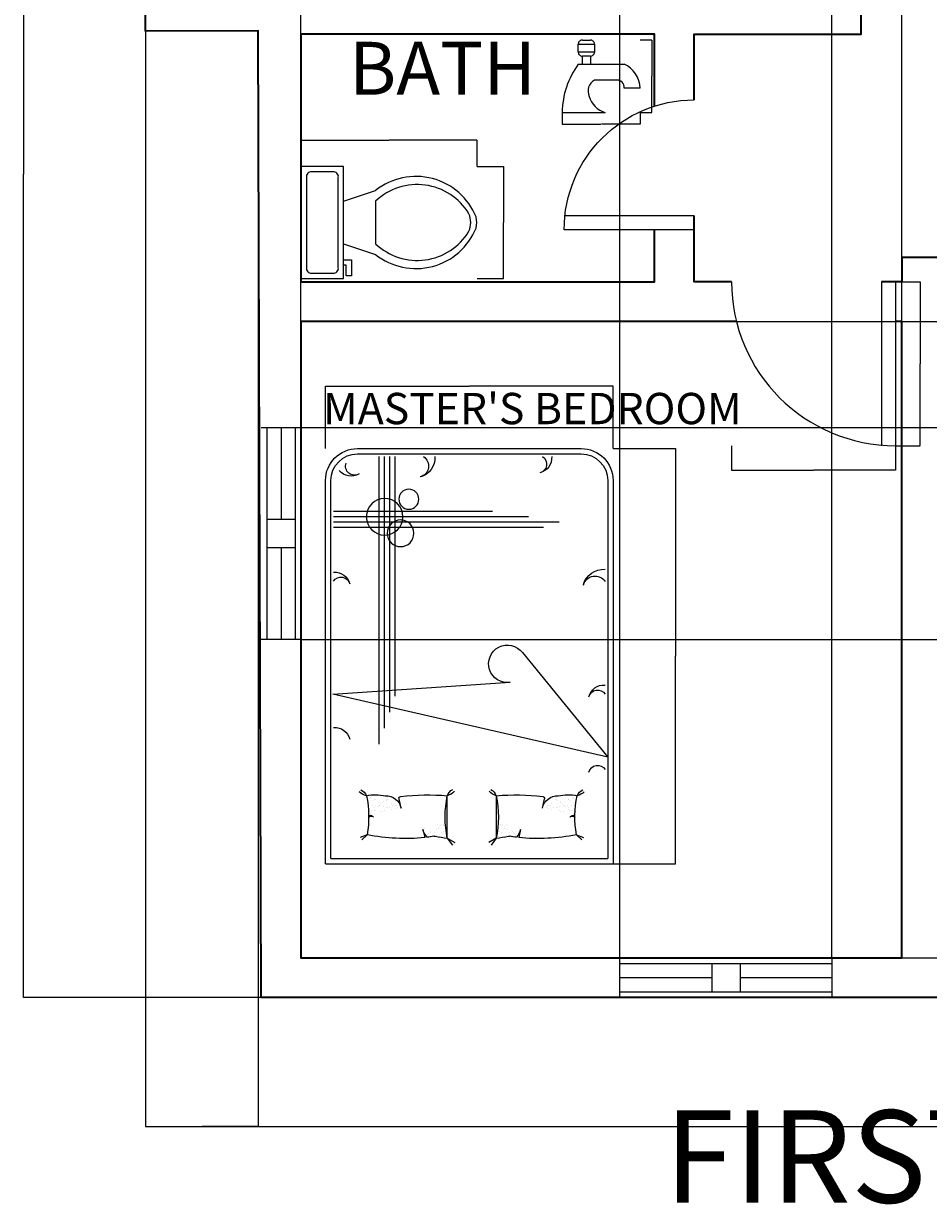
# Model space of a CAD drawing. Units: millimetres. Extents: x 19292 to 100733, y 12374 to 26974.
# Tile 19 of 24: x 42699 to 47819, y 12374 to 19054. Entities that reach past the tile are written whole.
import ezdxf

# ---------------------------------------------------------------- set-up
doc = ezdxf.new("R2010")
doc.units = ezdxf.units.MM
for name, color, linetype, lineweight in [('A-ANNO-DIMS', 2, 'Continuous', 18), ('A-ANNO-TEXT', 7, 'Continuous', 35), ('A-AREA-IDEN', 3, 'Continuous', 25), ('A-DOOR', 4, 'Continuous', 25), ('A-FLOR-FIXT', 9, 'Continuous', 18), ('A-FURN', 8, 'Continuous', 18), ('A-GLAZ', 3, 'Continuous', 25), ('A-WALL', 7, 'Continuous', 35)]:
    doc.layers.add(name, color=color, linetype=linetype, lineweight=lineweight)
doc.layers.add('FURNITURE', color=40, linetype='Continuous')
doc.layers.add('WINDOWS', color=50, linetype='Continuous')
doc.styles.get("Standard").update_dxf_attribs({"font": 'arial.ttf'})
doc.dimstyles.get("Standard").update_dxf_attribs({"dimtxt": 0.18, "dimasz": 0.18, "dimexe": 0.18, "dimexo": 0.0625, "dimgap": 0.09, "dimtad": 0, "dimtih": 1, "dimtoh": 1, "dimdec": 4, "dimzin": 0, "dimdsep": 46, "dimtxsty": 'Standard', "dimcen": 0.09, "dimadec": 0, "dimazin": 0, "dimtfac": 1, "dimtdec": 4, "dimtofl": 0, "dimtmove": 0, "dimatfit": 3, "dimfxl": 1, "dimtolj": 1, "dimtzin": 0, "dimarcsym": 0})

# ---------------------------------------------------------------- blocks, each defined once
blk = doc.blocks.new('DBED-4FT6')
at = {"layer": 'FURNITURE'}
for p, q in [((-27, 0), (-27, -72)), ((-27, 0), (26.99999999999997, 5.68e-14)), ((27, -72.00000000000023), (26.99999999999997, 5.68e-14)), ((-26, -1), (-26, -72)), ((-26, -1), (26.00000000000003, -0.9999999999997726)), ((26, -72.00000000000023), (26.00000000000003, -0.9999999999997726)), ((-4.134652103803261, -4.817063052123046), (-3.144796483066045, -3.500606371767958)), ((-4.134652103803261, -4.817063052122875), (-2.713769052616612, -3.999588591179417)), ((5.060678666421324, -4.817063052122875), (3.639795615234675, -3.999588591179417)), ((5.060678666421324, -4.817063052123046), (4.070823045684107, -3.500606371767958)), ((-19.18306202227052, -5.485972547936796), (-20.50060919072149, -4.967335516912726)), ((-19.18306202227052, -5.485972547936967), (-20.20772305100416, -4.498686779813965)), ((-8.713720467787255, -6.492365964457349), (-8.352181760678093, -4.952469549742318)), ((-8.40590424041818, -6.637378314066779), (-8.40590424041818, -6.637378314066779)), ((-8.239079784370745, -5.562538396824265), (-8.239079784370745, -5.562538396824265)), ((-7.82267294259384, -5.507717396091834), (-7.82267294259384, -5.507717396091834)), ((-7.611546033681406, -5.809807366600068), (-7.611546033681406, -5.809807366600068)), ((-7.515425131198753, -5.088011999378352), (-7.515425131198753, -5.088011999378352)), ((-7.374544898039516, -5.845988456355428), (-7.374544898039516, -5.845988456355428)), ((-7.367969663836447, -5.22313004090148), (-7.367969663836447, -5.22313004090148)), ((-7.274189455356292, -6.024727209938816), (-7.274189455356292, -6.024727209938816)), ((-6.736049374527851, -5.364660689418656), (-6.736049374527851, -5.364660689418656)), ((-6.571710140081449, -5.952767465126385), (-6.571710140081449, -5.952767465126385)), ((-6.245189668756381, -6.559531928114552), (-6.245189668756381, -6.559531928114552)), ((-6.085661545466621, -5.279035507322305), (-6.085661545466621, -5.279035507322305)), ((-5.875720334132552, -6.590524621115605), (-5.875720334132552, -6.590524621115605)), ((-5.669254703689716, -5.224214506589873), (-5.669254703689716, -5.224214506589873)), ((-5.280472006961815, -5.819278030439932), (-5.280472006961815, -5.819278030439932)), ((-5.120232544280042, -5.805280123770785), (-5.120232544280042, -5.805280123770785)), ((-4.782875965954929, -6.020199967109533), (-4.782875965954929, -6.020199967109533)), ((-4.582631135623728, -5.081157799916695), (-4.582631135623728, -5.081157799916695)), ((-4.249112664583094, -5.02788817272858), (-4.249112664583094, -5.02788817272858)), ((5.175139227201157, -5.027888172729319), (5.175139227201157, -5.027888172729319)), ((5.50865769824179, -5.081157799916638), (5.50865769824179, -5.081157799916638)), ((5.708902528572991, -6.020199967109817), (5.708902528572991, -6.020199967109817)), ((6.046259106898105, -5.805280123771126), (6.046259106898105, -5.805280123771126)), ((6.206498569579878, -5.819278030440671), (6.206498569579878, -5.819278030440671)), ((6.595281266307779, -5.224214506589817), (6.595281266307779, -5.224214506589817)), ((6.801746896750614, -6.590524621115321), (6.801746896750614, -6.590524621115321)), ((7.011688108084683, -5.279035507322305), (7.011688108084683, -5.279035507322305)), ((7.171216231373705, -6.559531928115234), (7.171216231373705, -6.559531928115234)), ((7.497736702698773, -5.952767465126157), (7.497736702698773, -5.952767465126157)), ((7.662075937145914, -5.364660689418599), (7.662075937145914, -5.364660689418599)), ((8.200216017975094, -6.024727209939328), (8.200216017975094, -6.024727209939328)), ((8.293996226453771, -5.223130040901196), (8.293996226453771, -5.223130040901196)), ((8.30057146065684, -5.84598845635628), (8.30057146065684, -5.84598845635628)), ((8.441451693816077, -5.088011999378068), (8.441451693816077, -5.088011999378068)), ((8.537572596300208, -5.80980736660058), (8.537572596300208, -5.80980736660058)), ((8.748699505211903, -5.507717396091777), (8.748699505211903, -5.507717396091777)), ((9.165106346988807, -5.562538396824265), (9.165106346988807, -5.562538396824265)), ((9.639747030405317, -6.492365964457349), (9.278208323295416, -4.952469549742318)), ((9.331930803035561, -6.637378314067632), (9.331930803035561, -6.637378314067632)), ((20.10908858488784, -5.485972547936967), (21.13374961362223, -4.498686779813965)), ((20.10908858488858, -5.485972547936796), (21.42663575333882, -4.967335516912726)), ((-5.998452499838663, -7.338874652100457), (-5.998452499838663, -7.338874652100457)), ((-5.728264866770928, -6.725642662638733), (-5.728264866770928, -6.725642662638733)), ((-5.688613537228434, -7.034850473630854), (-5.688613537228434, -7.034850473630854)), ((-5.348064670777432, -7.253249470004163), (-5.348064670777432, -7.253249470004163)), ((-5.230077320474265, -7.360737045650239), (-5.230077320474265, -7.360737045650239)), ((-4.93200534301593, -7.455280086863638), (-4.93200534301593, -7.455280086863638)), ((-4.931657828999789, -7.198428469271675), (-4.931657828999789, -7.198428469271675)), ((5.857684391617851, -7.198428469271505), (5.857684391617851, -7.198428469271505)), ((5.85803190563331, -7.455280086863353), (5.85803190563331, -7.455280086863353)), ((6.156103883091589, -7.360737045650921), (6.156103883091589, -7.360737045650921)), ((6.274091233394756, -7.253249470003993), (6.274091233394756, -7.253249470003993)), ((6.614640099846496, -7.034850473631365), (6.614640099846496, -7.034850473631365)), ((6.654291429388308, -6.725642662638449), (6.654291429388308, -6.725642662638449)), ((6.924479062455986, -7.338874652100287), (6.924479062455986, -7.338874652100287)), ((-18.77590810264172, -9.83900715250769), (-18.77590810264172, -9.83900715250769)), ((-18.7469186025819, -9.831933062623136), (-18.7469186025819, -9.831933062623136)), ((-18.59621655837128, -9.4634697248635), (-18.59621655837128, -9.4634697248635)), ((-18.43855152431661, -10.05392699584638), (-18.43855152431661, -10.05392699584638)), ((-18.181365058572, -11.01410595179413), (-18.181365058572, -11.01410595179413)), ((-17.90022675242233, -10.10122688085266), (-17.90022675242233, -10.10122688085266)), ((-17.75277128506002, -10.23634492237579), (-17.75277128506002, -10.23634492237579)), ((-17.73180625429978, -10.63313818015905), (-17.73180625429978, -10.63313818015905)), ((-17.53097722951077, -10.92848076969778), (-17.53097722951077, -10.92848076969778)), ((-17.11457038773386, -10.87365976896535), (-17.11457038773386, -10.87365976896535)), ((-16.95651176130502, -10.9659823466007), (-16.95651176130502, -10.9659823466007)), ((-16.85297560618875, -11.06405025953836), (-16.85297560618875, -11.06405025953836)), ((-16.70044691192106, -9.841748322447756), (-16.70044691192106, -9.841748322447756)), ((-16.2845946132411, -9.834479909678294), (-16.2845946132411, -9.834479909678294)), ((-16.02794681966861, -10.73060306229217), (-16.02794681966861, -10.73060306229217)), ((-15.94723803491598, -10.04939975301698), (-15.94723803491598, -10.04939975301698)), ((-15.57109168263798, -10.55529179420631), (-15.57109168263798, -10.55529179420631)), ((-15.37755899060738, -10.64497788019582), (-15.37755899060738, -10.64497788019582)), ((-14.96115214883048, -10.59015687946339), (-14.96115214883048, -10.59015687946339)), ((-14.55161047764721, -10.26384189465318), (-14.55161047764721, -10.26384189465318)), ((-14.36166211678738, -11.05952301670902), (-14.36166211678738, -11.05952301670902)), ((-13.87452858076449, -10.44710017279021), (-13.87452858076449, -10.44710017279021)), ((-13.85562067169906, -10.9015990506424), (-13.85562067169906, -10.9015990506424)), ((-13.70816520433675, -11.03671709216553), (-13.70816520433675, -11.03671709216553)), ((-13.52461999197714, -10.56510705403116), (-13.52461999197714, -10.56510705403116)), ((-12.80860301424707, -10.50441610444505), (-13.20654336081225, -12.19935747834682)), ((13.73462957686513, -10.50441610444505), (14.13256992343031, -12.19935747834682)), ((14.45064655459447, -10.56510705403201), (14.45064655459447, -10.56510705403201)), ((14.63419176695407, -11.03671709216536), (14.63419176695407, -11.03671709216536)), ((14.78164723431638, -10.90159905064223), (14.78164723431638, -10.90159905064223)), ((14.80055514338181, -10.44710017278998), (14.80055514338181, -10.44710017278998)), ((15.28768867940545, -11.05952301670942), (15.28768867940545, -11.05952301670942)), ((15.47763704026454, -10.26384189465307), (15.47763704026454, -10.26384189465307)), ((15.8871787114478, -10.59015687946316), (15.8871787114478, -10.59015687946316)), ((16.30358555322471, -10.64497788019565), (16.30358555322471, -10.64497788019565)), ((16.49711824525531, -10.55529179420722), (16.49711824525531, -10.55529179420722)), ((16.87326459753331, -10.04939975301738), (16.87326459753331, -10.04939975301738)), ((16.95397338228594, -10.73060306229195), (16.95397338228594, -10.73060306229195)), ((17.21062117585842, -9.834479909678635), (17.21062117585842, -9.834479909678635)), ((17.62647347453912, -9.841748322448382), (17.62647347453912, -9.841748322448382)), ((17.77900216880681, -11.06405025953882), (17.77900216880681, -11.06405025953882)), ((17.8825383239224, -10.96598234660052), (17.8825383239224, -10.96598234660052)), ((18.04059695035192, -10.87365976896512), (18.04059695035192, -10.87365976896512)), ((18.45700379212883, -10.92848076969761), (18.45700379212883, -10.92848076969761)), ((18.65783281691711, -10.63313818015967), (18.65783281691711, -10.63313818015967)), ((18.6787978476774, -10.23634492237556), (18.6787978476774, -10.23634492237556)), ((18.82625331503971, -10.10122688085243), (18.82625331503971, -10.10122688085243)), ((19.10739162119006, -11.01410595179391), (19.10739162119006, -11.01410595179391)), ((19.36457808693467, -10.05392699584672), (19.36457808693467, -10.05392699584672)), ((19.5222431209886, -9.463469724863273), (19.5222431209886, -9.463469724863273)), ((19.67294516519922, -9.831933062623932), (19.67294516519922, -9.831933062623932)), ((19.70193466525978, -9.839007152508032), (19.70193466525978, -9.839007152508032)), ((-18.69652391609435, -11.37339207783361), (-18.69652391609435, -11.37339207783361)), ((-18.66542323901467, -12.3058799545372), (-18.66542323901467, -12.3058799545372)), ((-18.6461292296068, -12.91485109304403), (-18.6461292296068, -12.91485109304403)), ((-18.51796777165236, -12.44099799606033), (-18.51796777165236, -12.44099799606033)), ((-18.12980541361923, -11.84228893838752), (-18.12980541361923, -11.84228893838752)), ((-17.79244883529407, -12.05720878172627), (-17.79244883529407, -12.05720878172627)), ((-17.68141156781223, -12.17459719536947), (-17.68141156781223, -12.17459719536947)), ((-17.44376818388207, -12.98831991447582), (-17.44376818388207, -12.98831991447582)), ((-16.79338035482089, -12.90269473237953), (-16.79338035482089, -12.90269473237953)), ((-16.65005222543351, -11.38320733765818), (-16.65005222543351, -11.38320733765818)), ((-16.59965753894596, -12.92466635286894), (-16.59965753894596, -12.92466635286894)), ((-16.37697351304393, -12.84787373164704), (-16.37697351304393, -12.84787373164704)), ((-16.26052195535686, -11.60373950258992), (-16.26052195535686, -11.60373950258992)), ((-16.11306648799456, -11.73885754411304), (-16.11306648799456, -11.73885754411304)), ((-15.63849192421787, -11.83776169555784), (-15.63849192421787, -11.83776169555784)), ((-15.52069699614969, -12.09675080941707), (-15.52069699614969, -12.09675080941707)), ((-15.31680696423956, -12.46849496833795), (-15.31680696423956, -12.46849496833795)), ((-15.3011353458927, -12.05268153889659), (-15.3011353458927, -12.05268153889659)), ((-15.29034994497795, -12.70481702497386), (-15.29034994497795, -12.70481702497386)), ((-14.55597933435581, -11.35649691174245), (-14.55597933435581, -11.35649691174245)), ((15.48200589697319, -11.35649691174331), (15.48200589697319, -11.35649691174331)), ((16.21637650759675, -12.70481702497392), (16.21637650759675, -12.70481702497392)), ((16.22716190851076, -12.05268153889693), (16.22716190851076, -12.05268153889693)), ((16.24283352685688, -12.46849496833772), (16.24283352685688, -12.46849496833772)), ((16.44672355876702, -12.09675080941792), (16.44672355876702, -12.09675080941792)), ((16.56451848683594, -11.83776169555824), (16.56451848683594, -11.83776169555824)), ((17.03909305061188, -11.73885754411276), (17.03909305061188, -11.73885754411276)), ((17.18654851797419, -11.60373950258963), (17.18654851797419, -11.60373950258963)), ((17.303000075662, -12.8478737316471), (17.303000075662, -12.8478737316471)), ((17.52568410156328, -12.92466635286979), (17.52568410156328, -12.92466635286979)), ((17.57607878805157, -11.38320733765908), (17.57607878805157, -11.38320733765908)), ((17.71940691743896, -12.90269473237953), (17.71940691743896, -12.90269473237953)), ((18.36979474650013, -12.98831991447588), (18.36979474650013, -12.98831991447588)), ((18.60743813042956, -12.17459719537038), (18.60743813042956, -12.17459719537038)), ((18.71847539791213, -12.05720878172661), (18.71847539791213, -12.05720878172661)), ((19.0558319762373, -11.84228893838792), (19.0558319762373, -11.84228893838792)), ((19.44399433426969, -12.4409979960601), (19.44399433426969, -12.4409979960601)), ((19.57215579222412, -12.91485109304494), (19.57215579222412, -12.91485109304494)), ((19.59144980163199, -12.30587995453698), (19.59144980163199, -12.30587995453698)), ((19.62255047871167, -11.37339207783429), (19.62255047871167, -11.37339207783429)), ((25.99999999999997, -20.04251490499428), (-25.62857142857144, -31.89664668985566)), ((9.968437092424097, -39.68281460107684), (25.99999999999997, -20.04251490499428)), ((-16.98298633143713, -76.49999999999977), (-16.98298633143804, -22.5)), ((-15.98298633143713, -76.49999999999977), (-15.98298633143804, -25.49999999999978)), ((-14.98298633143713, -76.49999999999977), (-14.98298633143804, -28.5)), ((-25.62857142857075, -31.89664668985566), (7.69367787486118, -34.10856123257989)), ((-13.98298633143713, -76.49999999999977), (-13.98298633143804, -31.5)), ((13.92237160184822, -63.18866900046464), (-25.5, -63.18866900046464)), ((16.878192650664, -64.18866900046464), (-25.5, -64.18866900046464)), ((11.10090459947105, -65.18866900046442), (-25.5, -65.18866900046464)), ((4.383130216417612, -66.18866900046442), (-25.5, -66.18866900046464)), ((-21, -77), (21, -77.0000000000002)), ((-21, -78), (21, -78.0000000000002))]:
    blk.add_line(p, q, dxfattribs=at)
for centre, radius in [((-12.91182106300494, -62.08454274520204), 2.504372971601696), ((-15.90739414396376, -65.18866900046464), 3.437232026160017), ((-11.36543750832788, -68.48173730478015), 1.878279728701272)]:
    blk.add_circle(centre, radius, dxfattribs=at)
for centre, radius, start, end in [((-39.10651142374138, -8.817063052122649), 20.20000000000147, 348.6069698988843, 9.491743103753544), ((-11.96490980142209, -41.81687628144138), 37.041008187906, 84.4028612645958, 101.2370836512883), ((-4.825879607851106, -7.608979000930446), 4.045013130436864, 139.9097590679286, 163.9755921234989), ((-11.52336853637479, -33.34663058587759), 28.57069839034993, 80.1409392097565, 82.7553866503384), ((-6.494365647111578, -4.409680956092984), 0.8, 260.1409392097565, 276.031827105606), ((-67.64177770808838, 360.6114736163754), 370.9058781068297, 279.5022474872839, 279.8588573948661), ((15.66534789619453, -8.817063052122135), 20.19999999999818, 168.5788137250011, 191.4211862750058), ((15.66534789619817, -8.817063052122649), 20.20000000000147, 168.5788137249941, 191.4211862750058), ((42751.26187429979, -8.817063056011648), 42755.39671351448, 179.9946396680611, 180.0053603319291), ((-14.73932133358011, -8.817063052122649), 20.20000000000147, 348.5788137249941, 11.42118627500586), ((-42750.33584773717, -8.817063056011648), 42755.39671351448, 359.9946396680676, 0.0053603319421324), ((-14.73932133357721, -8.817063052122135), 20.19999999999818, 348.5788137249941, 11.42118627499883), ((68.56780427070572, 360.6114736163754), 370.9058781068297, 260.141142605134, 260.4977525127162), ((7.420392209728902, -4.409680956092984), 0.8, 263.968172894394, 279.8590607902435), ((12.44939509899285, -33.34663058587759), 28.57069839034993, 97.2446133496616, 99.8590607902435), ((5.751906170469169, -7.608979000930446), 4.045013130436864, 16.0244078765011, 40.09024093207139), ((12.89093636403942, -41.81687628144138), 37.041008187906, 78.76291634871168, 95.59713873540417), ((40.03253798635941, -8.817063052122649), 20.20000000000147, 170.5082568962464, 191.3930301011157), ((-18.63439747950781, -8.362835026573748), 0.7823789253415179, 249.4968528373028, 325.7977956221763), ((-18.4002510232591, -8.445355047199143), 0.5460297530620258, 201.8040695959829, 319.1334346759098), ((19.32627758587716, -8.445355047199143), 0.5460297530620258, 220.8665653240902, 338.1959304040171), ((19.56042404212513, -8.362835026573748), 0.7823789253415179, 214.2022043778237, 290.5031471626973), ((-15.61384730787557, -9.916934814375791), 2.86610010521538, 266.7825255240543, 348.1719149754145), ((16.53987387049363, -9.916934814375791), 2.86610010521538, 191.8280850245854, 273.2174744759457), ((-18.77582684722529, -15.36188282958866), 2.608691937302173, 101.6935339662269, 136.5635486949323), ((-21.64959486574241, -11.66451602127745), 2.608691937302173, 299.1485263283325, 334.0185410570184), ((-17.59820796861624, -5.617120538590143), 7.389908305163763, 256.6498532633935, 284.285581023734), ((-12.81713200699761, -12.29078393797522), 0.4, 166.787330358343, 262.8769841008062), ((-7.849044883706142, 31.23309670203668), 44.20648468370187, 263.4825574665681, 274.8198866450032), ((-1.728460786103994, -11.80933443470422), 2.608691937302173, 202.7242534275457, 237.5942681562781), ((-4.807664589399962, -15.33744552666542), 2.608691937302173, 40.17924578964186, 75.04926051838007), ((5.733691152018025, -15.33744552666542), 2.608691937302173, 104.9507394816199, 139.8207542103581), ((2.654487348722057, -11.80933443470422), 2.608691937302173, 302.4057318437219, 337.2757465724543), ((8.775071446323466, 31.23309670203668), 44.20648468370187, 265.1801133549968, 276.5174425334318), ((13.74315856961567, -12.29078393797522), 0.4, 277.1230158991938, 13.21266964165692), ((18.52423453123356, -5.617120538590143), 7.389908305163763, 255.7144189762659, 283.3501467366066), ((19.70185340984335, -15.36188282958866), 2.608691937302173, 43.43645130506771, 78.3064660337731), ((22.57562142836048, -11.66451602127745), 2.608691937302173, 205.9814589429815, 240.8514736716675), ((24.08149477166717, -16.81385886181465), 1.693091563593251, 194.451540940981, 326.9105817271671), ((-25.2881588087821, -22.70588367900495), 2.933920970030247, 265.8594053605621, 345.9527428336846), ((24.08149477166717, -30.96393635208892), 1.693091563593251, 194.451540940981, 326.9105817271671), ((25.28815880878119, -30.6743386403075), 2.933920970030691, 194.0472571663257, 274.140594639438), ((7.144201548013711, -37.58406550475044), 3.518672218272346, 81.0159135592615, 323.3831798465962), ((-25.28815880878119, -51.86055593582091), 2.933920970030691, 265.8594053605621, 345.9527428336743), ((-24.08149477166717, -52.15015364760233), 1.693091563593251, 213.0894182728328, 345.548459059019), ((23.60865969555653, -51.81050935983859), 2.257455418124377, 194.451540940981, 326.9105817271699), ((25.21754507837523, -51.42437907746352), 3.911894626707589, 194.0472571663257, 274.140594639438), ((-21, -72), 6, 180, 270), ((-21, -72), 5, 180, 270), ((-22.19032021997464, -75.74024097389656), 2.933920970030691, 59.04725716631266, 140.6216534048161), ((-21.541856402534, -74.6822241448225), 1.69309156359317, 59.45154094095176, 200.6983000057678), ((-9.760470192471985, -74.7268684645835), 2.116364454491481, 303.0894182728446, 75.5484590590127), ((-10.12246733219854, -76.23519851097626), 3.667401212538364, 355.8594053605848, 75.95274283367745), ((21, -72.00000000000023), 5, 270, 0), ((21, -72.00000000000023), 6, 270, 0), ((12.54583364175596, -76.28815880878142), 2.933920970030691, 355.8594053605848, 75.95274283367745), ((12.83543135353738, -75.081494771667), 1.693091563593251, 303.0894182728446, 75.5484590590127)]:
    blk.add_arc(centre, radius, start, end, dxfattribs=at)
blk = doc.blocks.new('TAP-SIDELEV')
for p, q in [((0.9999853785046433, 4.25000541523623), (1.999985378504643, 4.25000541523623)), ((1.999985378504643, 3.75000541523623), (0.9999853785046433, 3.75000541523623)), ((0.9999853785046433, 3.00000541523623), (3.840125540729427, 3.00000541523623)), ((1.249985378504643, 3.00000541523623), (1.249985378504643, 3.50000541523623)), ((1.749985378504643, 3.50000541523623), (1.749985378504643, 3.00000541523623)), ((3.527288395467852, 2.00000541523623), (1.999985378504643, 2.00000541523623)), ((4.840309954143972, 1.50000541523623), (3.840309954143972, 1.50000541523623)), ((-1.46214953567e-05, 5.415236231e-06), (0.2499853785046433, 5.415236231e-06)), ((0.2499853785046433, 5.415236231e-06), (2.675565113506539, 5.415236231e-06))]:
    blk.add_line(p, q)
for points in [[(1.249985378504643, 4.50000541523623), (1.749985378504643, 4.50000541523623)], [(0.9999853785046433, 3.75000541523623), (0.9999853785046433, 4.25000541523623)], [(1.999985378504643, 4.25000541523623), (1.999985378504643, 3.75000541523623)], [(1.749985378504643, 3.50000541523623), (1.249985378504643, 3.50000541523623)]]:
    blk.add_lwpolyline(points)
for centre, radius, start, end in [((1.242385378504675, 4.257505415236281), 0.2425917, 88.22243000000017, 181.7776), ((1.757485378504636, 4.257505415236281), 0.2425917, 358.2224, 91.77756999999983), ((1.242385378504675, 3.742405415236319), 0.2425917, 178.2223999999999, 271.7775999999998), ((1.757485378504636, 3.742405415236319), 0.2425917, 268.2224000000001, 1.777565000000075), ((5.084285378504628, -0.0280945847637639), 5.084362999999999, 143.4467, 179.6834000000001), ((3.172409954143997, 1.471305415236273), 1.668163, 0.9827694999999721, 66.40494208784), ((2.37686141733268, 1.325114461238403), 0.7729898760208992, 119.180086595352, 204.871573560288), ((3.433909954144009, 1.593605415236268), 0.4169898, 347.0191999999999, 102.9807999999998), ((3.050564044119678, 1.37500541523623), 1.425219, 195.2551000000002, 254.7449000000001)]:
    blk.add_arc(centre, radius, start, end)
blk = doc.blocks.new('WC01')
at = {"layer": 'FURNITURE'}
for p, q in [((10.5, 0), (-10.5, 0)), ((-10.5, 0), (-10.5, -8)), ((10.5, -8), (10.5, 0)), ((-9.5, -2), (-9.5, -6)), ((8.5, -1), (-8.5, -1)), ((9.5, -6), (9.5, -2)), ((-10.5, -8), (10.5, -8)), ((-10, -9.5), (-10, -8.5)), ((-10, -8.5), (-8, -8.5)), ((-8.5, -7), (8.5, -7)), ((-8, -8.5), (-8, -8)), ((-7, -8), (-7, -9.5)), ((-4, -8), (-6, -14)), ((4, -8), (6, -14)), ((-7, -9.5), (-10, -9.5)), ((4, -14), (-4, -14))]:
    blk.add_line(p, q, dxfattribs=at)
for centre, radius, start, end in [((-8.625, -1.875), 0.8838834999999999, 81.86989999999966, 188.1301000000003), ((8.625, -1.875), 0.8838834999999999, 351.8698999999996, 98.13010000000035), ((-8.625, -6.125), 0.8838834999999999, 171.8698980000006, 278.1301000000004), ((8.625, -6.125), 0.8838834999999999, 261.8698999999996, 8.13010000000033), ((3.519562435188959, -21.58049502388982), 12.16902005083646, 141.4691096810951, 247.9714346835572), ((4.199957580658804, -21.81740929088454), 11.3291791325804, 136.3677254423712, 238.9468239374052), ((-3.519499936778316, -21.58047137067521), 12.16903423757823, 292.0284332733146, 38.5307063680049), ((-4.199890672038463, -21.81738596564128), 11.32918622148567, 301.0530065773862, 43.6320921669473), ((2.09660981625e-05, -27.87646475467881), 4, 245.7318247449368, 294.2681740488958), ((2.09415214272e-05, -28.99996806116076), 4, 254.8605283244431, 285.1394707718437)]:
    blk.add_arc(centre, radius, start, end, dxfattribs=at)
blk = doc.blocks.new('WW')
at = {"layer": 'WINDOWS'}
for p, q in [((-5183.867826392408, -4940.876860268414), (-3983.867826392409, -4940.876860268414)), ((-4663.867826392415, -4940.876860268414), (-4663.867826392408, -5100.876860268415)), ((-4503.867826392416, -4940.876860268414), (-4503.867826392408, -5100.876860268415)), ((-4503.867826392416, -4940.876860268414), (-4503.867826392408, -5100.876860268415)), ((-5183.867826392408, -5020.876860268414), (-4663.867826392408, -5020.876860268415)), ((-4503.867826392416, -5020.876860268414), (-3983.867826392409, -5020.876860268414)), ((-5183.867826392408, -5100.876860268414), (-3983.867826392409, -5100.876860268414))]:
    blk.add_line(p, q, dxfattribs=at)
for points in [[(-5183.867826392408, -5133.376860268413), (-5183.867826392408, -4908.376860268414)], [(-3983.867826392409, -4908.376860268414), (-3983.867826392409, -5133.376860268413)]]:
    blk.add_lwpolyline(points, dxfattribs=at)
blk = doc.blocks.new('DOOR-750')
for p, q in [((655.272448405085, -6.32018709439e-05), (655.272448405085, 735.2719952907646)), ((735.272448405085, -6.32018709439e-05), (735.272448405085, 735.2719952907646)), ((735.272448405085, -6.32018709439e-05), (655.272448405085, -6.32018709439e-05)), ((735.272448405085, -6.32018709439e-05), (655.272448405085, -6.32018709439e-05))]:
    blk.add_line(p, q)
blk.add_arc((735.272448405085, -6.32018709439e-05), 735.2720584926371, 90, 180)
blk = doc.blocks.new('DOOR-SWING-900')
blk.add_line((927.6985029579554, 927.698603252542), (927.6985029579554, -0.0001625114309718))
blk.add_arc((927.6985029579554, 927.698603252542), 927.6987657639734, 180, 270)
blk = doc.blocks.new('*D24')
at = {"layer": 'A-ANNO-DIMS', "color": 0, "lineweight": -2, "transparency": 16777216}
for p, q in [((46034.63806935272, 16650.17552620515), (46387.30813187039, 16650.17552620515)), ((46387.12813187039, 16649.99552620515), (46387.1281318704, 15475.1835101731)), ((46387.1281318704, 14300.00510942071), (46387.1281318704, 15474.81712545277)), ((46034.63806935272, 14299.82510942071), (46387.3081318704, 14299.82510942071))]:
    blk.add_line(p, q, dxfattribs=at)
at = {"layer": 'A-ANNO-DIMS', "color": 0, "transparency": 16777216}
for points in [[(46387.09813187039, 16649.99552620515), (46387.15813187038, 16649.99552620515), (46387.12813187039, 16650.17552620515)], [(46387.09813187039, 14300.00510942071), (46387.15813187039, 14300.00510942071), (46387.1281318704, 14299.82510942071)]]:
    blk.add_solid(points, dxfattribs=at)
at = {"layer": 'Defpoints', "color": 0, "transparency": 16777216}
for p in [(46034.57556935271, 16650.17552620515), (46034.57556935271, 14299.82510942071), (46387.1281318704, 14299.82510942071)]:
    blk.add_point(p, dxfattribs=at)
at = {"layer": 'A-ANNO-DIMS', "color": 0, "transparency": 16777216, "insert": (46387.12813187039, 15475.00031781291), "char_height": 0.18, "attachment_point": 5}
blk.add_mtext('\\A1;DOUBLE BED 2350 TYP.', dxfattribs=at)
blk = doc.blocks.new('*D25')
at = {"layer": 'A-ANNO-DIMS', "color": 0, "lineweight": -2, "transparency": 16777216}
for p, q in [((44407.40989619425, 16650.23802620514), (44407.40989619425, 17002.90808872281)), ((44407.58989619425, 17002.72808872281), (45220.3332648335, 17002.72808872281)), ((46034.3955693527, 17002.72808872281), (45221.65220071345, 17002.72808872281)), ((46034.5755693527, 16650.23802620514), (46034.5755693527, 17002.90808872281))]:
    blk.add_line(p, q, dxfattribs=at)
at = {"layer": 'A-ANNO-DIMS', "color": 0, "transparency": 16777216}
for points in [[(44407.58989619425, 17002.75808872281), (44407.58989619425, 17002.69808872281), (44407.40989619425, 17002.72808872281)], [(46034.3955693527, 17002.75808872281), (46034.3955693527, 17002.69808872281), (46034.5755693527, 17002.72808872281)]]:
    blk.add_solid(points, dxfattribs=at)
at = {"layer": 'Defpoints', "color": 0, "transparency": 16777216}
for p in [(46034.5755693527, 17002.72808872281), (44407.40989619425, 16650.17552620514), (46034.5755693527, 16650.17552620514)]:
    blk.add_point(p, dxfattribs=at)
at = {"layer": 'A-ANNO-DIMS', "color": 0, "transparency": 16777216, "insert": (45220.99273277348, 17002.72808872281), "char_height": 0.18, "attachment_point": 5}
blk.add_mtext('\\A1;1627 TYP.', dxfattribs=at)
blk = doc.blocks.new('*D28')
at = {"layer": 'A-ANNO-DIMS', "color": 0, "lineweight": -2, "transparency": 16777216}
for p, q in [((47632.94877694873, 17593.99260027244), (47772.22109181335, 17593.99260027244)), ((47772.04109181335, 17593.81260027244), (47772.04109181335, 17130.32634835907)), ((47772.04109181335, 16666.47383450846), (47772.04109181335, 17129.96008642183)), ((47632.94877694873, 16666.29383450846), (47772.22109181335, 16666.29383450846))]:
    blk.add_line(p, q, dxfattribs=at)
at = {"layer": 'A-ANNO-DIMS', "color": 0, "transparency": 16777216}
for points in [[(47772.01109181334, 17593.81260027244), (47772.07109181334, 17593.81260027244), (47772.04109181335, 17593.99260027244)], [(47772.01109181334, 16666.47383450846), (47772.07109181334, 16666.47383450846), (47772.04109181335, 16666.29383450846)]]:
    blk.add_solid(points, dxfattribs=at)
at = {"layer": 'Defpoints', "color": 0, "transparency": 16777216}
for p in [(47632.88627694873, 17593.99260027244), (47772.04109181335, 17593.99260027244), (47632.88627694873, 16666.29383450846)]:
    blk.add_point(p, dxfattribs=at)
at = {"layer": 'A-ANNO-DIMS', "color": 0, "transparency": 16777216, "insert": (47772.04109181335, 17130.14321739043), "char_height": 0.18, "attachment_point": 5}
blk.add_mtext('\\A1;DOOR 900 928 TYP.', dxfattribs=at)
blk = doc.blocks.new('*D29')
at = {"layer": 'A-ANNO-DIMS', "color": 0, "lineweight": -2, "transparency": 16777216}
for p, q in [((46705.18751118475, 16666.23133450846), (46705.18751118475, 16526.95901964386)), ((47632.88627694872, 16666.23133450846), (47632.88627694872, 16526.95901964386)), ((46705.36751118476, 16527.13901964386), (47168.43887905992, 16527.13901964386)), ((47632.70627694871, 16527.13901964386), (47169.63490907356, 16527.13901964386))]:
    blk.add_line(p, q, dxfattribs=at)
at = {"layer": 'A-ANNO-DIMS', "color": 0, "transparency": 16777216}
for points in [[(46705.36751118476, 16527.16901964386), (46705.36751118476, 16527.10901964386), (46705.18751118475, 16527.13901964386)], [(47632.70627694871, 16527.16901964386), (47632.70627694871, 16527.10901964386), (47632.88627694872, 16527.13901964386)]]:
    blk.add_solid(points, dxfattribs=at)
at = {"layer": 'Defpoints', "color": 0, "transparency": 16777216}
for p in [(46705.18751118475, 16666.29383450846), (47632.88627694872, 16666.29383450846), (47632.88627694872, 16527.13901964386)]:
    blk.add_point(p, dxfattribs=at)
at = {"layer": 'A-ANNO-DIMS', "color": 0, "transparency": 16777216, "insert": (47169.03689406674, 16527.13901964386), "char_height": 0.18, "attachment_point": 5}
blk.add_mtext('\\A1;928 TYP.', dxfattribs=at)
blk = doc.blocks.new('*D38')
at = {"layer": 'A-ANNO-DIMS', "color": 0, "lineweight": -2, "transparency": 16777216}
for p, q in [((44268.67420168258, 18245.59675392526), (44268.67420168258, 18395.08012642252)), ((44268.85420168257, 18394.90012642252), (44765.71434511363, 18394.90012642252)), ((45264.26668499762, 18394.90012642252), (44767.40654156657, 18394.90012642252)), ((45264.44668499763, 18245.59675392526), (45264.44668499763, 18395.08012642252))]:
    blk.add_line(p, q, dxfattribs=at)
at = {"layer": 'A-ANNO-DIMS', "color": 0, "transparency": 16777216}
for points in [[(44268.85420168257, 18394.93012642252), (44268.85420168257, 18394.87012642252), (44268.67420168258, 18394.90012642252)], [(45264.26668499762, 18394.93012642252), (45264.26668499762, 18394.87012642252), (45264.44668499763, 18394.90012642252)]]:
    blk.add_solid(points, dxfattribs=at)
at = {"layer": 'Defpoints', "color": 0, "transparency": 16777216}
for p in [(44268.67420168258, 18394.90012642252), (44268.67420168258, 18245.53425392526), (45264.44668499763, 18245.53425392526)]:
    blk.add_point(p, dxfattribs=at)
at = {"layer": 'A-ANNO-DIMS', "color": 0, "transparency": 16777216, "insert": (44766.5604433401, 18394.90012642252), "char_height": 0.18, "attachment_point": 5}
blk.add_mtext('\\A1;WC 996 TYP.', dxfattribs=at)
blk = doc.blocks.new('*D39')
at = {"layer": 'A-ANNO-DIMS', "color": 0, "lineweight": -2, "transparency": 16777216}
for p, q in [((45264.50918499764, 18245.53425392527), (45413.99255749491, 18245.53425392527)), ((45413.81255749492, 18245.35425392527), (45413.81255749492, 17929.32289311824)), ((45413.81255749492, 17612.92760325254), (45413.81255749492, 17928.95896405957)), ((45264.50918499764, 17612.74760325254), (45413.99255749491, 17612.74760325254))]:
    blk.add_line(p, q, dxfattribs=at)
at = {"layer": 'A-ANNO-DIMS', "color": 0, "transparency": 16777216}
for points in [[(45413.78255749491, 18245.35425392527), (45413.84255749491, 18245.35425392527), (45413.81255749492, 18245.53425392527)], [(45413.78255749491, 17612.92760325254), (45413.84255749491, 17612.92760325254), (45413.81255749492, 17612.74760325254)]]:
    blk.add_solid(points, dxfattribs=at)
at = {"layer": 'Defpoints', "color": 0, "transparency": 16777216}
for p in [(45264.44668499764, 18245.53425392527), (45413.81255749492, 18245.53425392527), (45264.44668499764, 17612.74760325254)]:
    blk.add_point(p, dxfattribs=at)
at = {"layer": 'A-ANNO-DIMS', "color": 0, "transparency": 16777216, "insert": (45413.81255749492, 17929.14092858889), "char_height": 0.18, "attachment_point": 5}
blk.add_mtext('\\A1;633 TYP.', dxfattribs=at)
blk = doc.blocks.new('*D40')
at = {"layer": 'A-ANNO-DIMS', "color": 0, "lineweight": -2, "transparency": 16777216}
for p, q in [((45746.8110979714, 18551.75783262261), (45746.8110979714, 18485.54556456821)), ((46187.44288500068, 18551.75783262261), (46187.44288500068, 18485.54556456821)), ((45746.9910979714, 18485.72556456821), (45965.70092736599, 18485.72556456821)), ((46187.26288500068, 18485.72556456821), (45968.5530556061, 18485.72556456821))]:
    blk.add_line(p, q, dxfattribs=at)
at = {"layer": 'A-ANNO-DIMS', "color": 0, "transparency": 16777216}
for points in [[(45746.9910979714, 18485.75556456821), (45746.9910979714, 18485.69556456822), (45746.8110979714, 18485.72556456821)], [(46187.26288500068, 18485.75556456821), (46187.26288500068, 18485.69556456822), (46187.44288500068, 18485.72556456821)]]:
    blk.add_solid(points, dxfattribs=at)
at = {"layer": 'Defpoints', "color": 0, "transparency": 16777216}
for p in [(45746.8110979714, 18551.82033262261), (46187.44288500068, 18551.82033262261), (46187.44288500068, 18485.72556456821)]:
    blk.add_point(p, dxfattribs=at)
at = {"layer": 'A-ANNO-DIMS', "color": 0, "transparency": 16777216, "insert": (45967.12699148604, 18485.72556456821), "char_height": 0.18, "attachment_point": 5}
blk.add_mtext('\\A1;WASH BASIN 441 TYP.', dxfattribs=at)
blk = doc.blocks.new('*D41')
at = {"layer": 'A-ANNO-DIMS', "color": 0, "lineweight": -2, "transparency": 16777216}
for p, q in [((46187.5053850007, 18961.65695604733), (46253.7176530551, 18961.65695604733)), ((46253.53765305511, 18961.47695604733), (46253.53765305511, 18756.92054747276)), ((46253.53765305511, 18552.00033262262), (46253.53765305511, 18756.55674119719)), ((46187.5053850007, 18551.82033262262), (46253.7176530551, 18551.82033262262))]:
    blk.add_line(p, q, dxfattribs=at)
at = {"layer": 'A-ANNO-DIMS', "color": 0, "transparency": 16777216}
for points in [[(46253.50765305511, 18961.47695604733), (46253.5676530551, 18961.47695604733), (46253.53765305511, 18961.65695604733)], [(46253.50765305511, 18552.00033262262), (46253.5676530551, 18552.00033262262), (46253.53765305511, 18551.82033262262)]]:
    blk.add_solid(points, dxfattribs=at)
at = {"layer": 'Defpoints', "color": 0, "transparency": 16777216}
for p in [(46187.4428850007, 18961.65695604733), (46253.53765305511, 18961.65695604733), (46187.4428850007, 18551.82033262262)]:
    blk.add_point(p, dxfattribs=at)
at = {"layer": 'A-ANNO-DIMS', "color": 0, "transparency": 16777216, "insert": (46253.53765305511, 18756.73864433496), "char_height": 0.18, "attachment_point": 5}
blk.add_mtext('\\A1;410 TYP.', dxfattribs=at)
blk = doc.blocks.new('*D100')
at = {"layer": 'A-ANNO-DIMS', "color": 0, "lineweight": -2, "transparency": 16777216}
for p, q in [((43388.92950300001, 22860.72493700001), (42698.81200300003, 22860.72493700001)), ((42698.99200300002, 22860.54493700001), (42698.99200300002, 18202.54073302934)), ((42698.99200300003, 13544.17260000001), (42698.99200300002, 18202.17680397067)), ((44043.61170200002, 13543.9926), (42698.81200300003, 13543.9926))]:
    blk.add_line(p, q, dxfattribs=at)
at = {"layer": 'A-ANNO-DIMS', "color": 0, "transparency": 16777216}
for points in [[(42698.96200300003, 22860.54493700001), (42699.02200300003, 22860.54493700001), (42698.99200300002, 22860.72493700001)], [(42698.96200300004, 13544.17260000001), (42699.02200300003, 13544.17260000001), (42698.99200300003, 13543.9926)]]:
    blk.add_solid(points, dxfattribs=at)
at = {"layer": 'Defpoints', "color": 0, "transparency": 16777216}
for p in [(43388.99200300001, 22860.72493700001), (42698.99200300003, 13543.9926), (44043.67420200001, 13543.9926)]:
    blk.add_point(p, dxfattribs=at)
at = {"layer": 'A-ANNO-DIMS', "color": 0, "transparency": 16777216, "insert": (42698.99200300002, 18202.35876849999), "char_height": 0.18, "attachment_point": 5}
blk.add_mtext('\\A1;9317', dxfattribs=at)
blk = doc.blocks.new('*D103')
at = {"layer": 'A-ANNO-DIMS', "color": 0, "lineweight": -2, "transparency": 16777216}
for p, q in [((44268.04262900001, 15568.9926), (57530.22278900005, 15568.99260000001)), ((57530.04278900005, 15568.81260000001), (57530.04278900005, 14669.1745031378)), ((57530.04278900005, 13769.17260000001), (57530.04278900005, 14668.81069686222)), ((44268.04262900001, 13768.9926), (57530.22278900005, 13768.99260000001))]:
    blk.add_line(p, q, dxfattribs=at)
at = {"layer": 'A-ANNO-DIMS', "color": 0, "transparency": 16777216}
for points in [[(57530.01278900006, 15568.81260000001), (57530.07278900005, 15568.81260000001), (57530.04278900005, 15568.99260000001)], [(57530.01278900006, 13769.17260000001), (57530.07278900005, 13769.17260000001), (57530.04278900005, 13768.99260000001)]]:
    blk.add_solid(points, dxfattribs=at)
at = {"layer": 'Defpoints', "color": 0, "transparency": 16777216}
for p in [(44267.98012900001, 15568.9926), (57530.04278900005, 15568.99260000001), (44267.98012900001, 13768.9926)]:
    blk.add_point(p, dxfattribs=at)
at = {"layer": 'A-ANNO-DIMS', "color": 0, "transparency": 16777216, "insert": (57530.04278900004, 14668.99259999999), "char_height": 0.18, "attachment_point": 5}
blk.add_mtext('\\A1;1800', dxfattribs=at)
blk = doc.blocks.new('*D104')
at = {"layer": 'A-ANNO-DIMS', "color": 0, "lineweight": -2, "transparency": 16777216}
for p, q in [((44268.04262900001, 17368.99260000001), (57530.22278900005, 17368.99260000001)), ((57530.04278900005, 17368.81260000001), (57530.04278900005, 17069.1745031378)), ((57530.04278900005, 16769.17260000001), (57530.04278900005, 17068.81069686222)), ((44268.04262900001, 16768.99260000001), (57530.22278900005, 16768.99260000001))]:
    blk.add_line(p, q, dxfattribs=at)
at = {"layer": 'A-ANNO-DIMS', "color": 0, "transparency": 16777216}
for points in [[(57530.01278900006, 17368.81260000001), (57530.07278900005, 17368.81260000001), (57530.04278900005, 17368.99260000001)], [(57530.01278900006, 16769.17260000001), (57530.07278900005, 16769.17260000001), (57530.04278900005, 16768.99260000001)]]:
    blk.add_solid(points, dxfattribs=at)
at = {"layer": 'Defpoints', "color": 0, "transparency": 16777216}
for p in [(44267.98012900001, 17368.99260000001), (57530.04278900005, 17368.99260000001), (44267.98012900001, 16768.99260000001)]:
    blk.add_point(p, dxfattribs=at)
at = {"layer": 'A-ANNO-DIMS', "color": 0, "transparency": 16777216, "insert": (57530.04278900005, 17068.99259999999), "char_height": 0.18, "attachment_point": 5}
blk.add_mtext('\\A1;600', dxfattribs=at)
blk = doc.blocks.new('*D112')
at = {"layer": 'A-ANNO-DIMS', "color": 0, "lineweight": -2, "transparency": 16777216}
for p, q in [((43388.992003, 22860.662437), (43388.992003, 12813.8126)), ((56840.04278899999, 15985.662601), (56840.04278899999, 12813.8126)), ((43389.172003, 12813.9926), (50114.11454470395, 12813.9926)), ((56839.86278899999, 12813.9926), (50114.92024729603, 12813.9926))]:
    blk.add_line(p, q, dxfattribs=at)
at = {"layer": 'A-ANNO-DIMS', "color": 0, "transparency": 16777216}
for points in [[(43389.172003, 12814.0226), (43389.172003, 12813.9626), (43388.992003, 12813.9926)], [(56839.86278899999, 12814.0226), (56839.86278899999, 12813.9626), (56840.04278899999, 12813.9926)]]:
    blk.add_solid(points, dxfattribs=at)
at = {"layer": 'Defpoints', "color": 0, "transparency": 16777216}
for p in [(43388.992003, 22860.724937), (56840.04278899999, 15985.725101), (56840.04278899999, 12813.9926)]:
    blk.add_point(p, dxfattribs=at)
at = {"layer": 'A-ANNO-DIMS', "color": 0, "transparency": 16777216, "insert": (50114.517396, 12813.9926), "char_height": 0.18, "attachment_point": 5}
blk.add_mtext('\\A1;13451', dxfattribs=at)
blk = doc.blocks.new('*D113')
at = {"layer": 'A-ANNO-DIMS', "color": 0, "lineweight": -2, "transparency": 16777216}
for p, q in [((43388.992003, 19010.662437), (43388.992003, 12813.8126)), ((44026.778429, 19012.632903), (44026.778429, 12813.8126)), ((43389.172003, 12813.9926), (43707.49083673669, 12813.9926)), ((44026.598429, 12813.9926), (43708.27959526329, 12813.9926))]:
    blk.add_line(p, q, dxfattribs=at)
at = {"layer": 'A-ANNO-DIMS', "color": 0, "transparency": 16777216}
for points in [[(43389.172003, 12814.0226), (43389.172003, 12813.9626), (43388.992003, 12813.9926)], [(44026.598429, 12814.0226), (44026.598429, 12813.9626), (44026.778429, 12813.9926)]]:
    blk.add_solid(points, dxfattribs=at)
at = {"layer": 'Defpoints', "color": 0, "transparency": 16777216}
for p in [(43388.992003, 19010.724937), (44026.778429, 19012.695403), (44026.778429, 12813.9926)]:
    blk.add_point(p, dxfattribs=at)
at = {"layer": 'A-ANNO-DIMS', "color": 0, "transparency": 16777216, "insert": (43707.88521599999, 12813.9926), "char_height": 0.18, "attachment_point": 5}
blk.add_mtext('\\A1;637.8', dxfattribs=at)
blk = doc.blocks.new('*D114')
at = {"layer": 'A-ANNO-DIMS', "color": 0, "lineweight": -2, "transparency": 16777216}
for p, q in [((44267.980129, 13769.0551), (44267.980129, 23550.904937)), ((44268.160129, 23550.724937), (45170.14306305662, 23550.724937)), ((46072.82794799999, 23550.724937), (45170.84501394339, 23550.724937)), ((46073.007948, 13769.0551), (46073.007948, 23550.904937))]:
    blk.add_line(p, q, dxfattribs=at)
at = {"layer": 'A-ANNO-DIMS', "color": 0, "transparency": 16777216}
for points in [[(44268.160129, 23550.754937), (44268.160129, 23550.694937), (44267.980129, 23550.724937)], [(46072.82794799999, 23550.754937), (46072.82794799999, 23550.694937), (46073.007948, 23550.724937)]]:
    blk.add_solid(points, dxfattribs=at)
at = {"layer": 'Defpoints', "color": 0, "transparency": 16777216}
for p in [(46073.007948, 23550.724937), (44267.980129, 13768.9926), (46073.007948, 13768.9926)]:
    blk.add_point(p, dxfattribs=at)
at = {"layer": 'A-ANNO-DIMS', "color": 0, "transparency": 16777216, "insert": (45170.4940385, 23550.724937), "char_height": 0.18, "attachment_point": 5}
blk.add_mtext('\\A1;1805', dxfattribs=at)
blk = doc.blocks.new('*D115')
at = {"layer": 'A-ANNO-DIMS', "color": 0, "lineweight": -2, "transparency": 16777216}
for p, q in [((47273.00794799999, 13769.0551), (47273.00794799999, 23550.904937)), ((47273.187948, 23550.724937), (47470.2045773813, 23550.724937)), ((47667.800129, 23550.724937), (47470.78349961869, 23550.724937)), ((47667.980129, 13769.0551), (47667.980129, 23550.904937))]:
    blk.add_line(p, q, dxfattribs=at)
at = {"layer": 'A-ANNO-DIMS', "color": 0, "transparency": 16777216}
for points in [[(47273.187948, 23550.754937), (47273.187948, 23550.694937), (47273.00794799999, 23550.724937)], [(47667.800129, 23550.754937), (47667.800129, 23550.694937), (47667.980129, 23550.724937)]]:
    blk.add_solid(points, dxfattribs=at)
at = {"layer": 'Defpoints', "color": 0, "transparency": 16777216}
for p in [(47667.980129, 23550.724937), (47273.00794799999, 13768.9926), (47667.980129, 13768.9926)]:
    blk.add_point(p, dxfattribs=at)
at = {"layer": 'A-ANNO-DIMS', "color": 0, "transparency": 16777216, "insert": (47470.4940385, 23550.724937), "char_height": 0.18, "attachment_point": 5}
blk.add_mtext('\\A1;395', dxfattribs=at)

msp = doc.modelspace()

# ---------------------------------------------------------------- linework, layer by layer
at = {"layer": 'A-DOOR'}
msp.add_line((47552.88627694873, 17593.99260027244), (47552.88627694873, 16666.29383450847), dxfattribs=at)
at = {"layer": 'A-WALL'}
for points in [[(43388.99200290092, 22860.72493679813), (49063.99200290092, 22860.72493679813), (49063.99200290092, 22460.72493679813), (56838.99200290092, 22460.72493679813), (56840.04278867613, 15985.72510139728), (54414.5194911604, 15985.331478935), (54414.5194911604, 14906.40305703235), (52089.65806670906, 14906.40305703235), (52089.65806670906, 13543.99260027244), (44043.67420168258, 13543.99260027244), (44026.77842884958, 19012.69540309651), (43388.99200290092, 19010.72493679813), (43388.99200290092, 22860.72493679813)], [(46492.98012915374, 18622.46175558771), (46492.98012915374, 18993.99260027244), (47438.99200290092, 18993.99260027244), (47438.99200290092, 19315.72493679813)], [(46267.98012915374, 18587.18969709507), (46267.98012915374, 18993.99260027244), (44267.98012915374, 18993.99260027244), (44267.98012915374, 17593.99260027244), (46267.98012915374, 17593.99260027244), (46267.98012915374, 17887.18969709508)], [(46705.18751118475, 17593.99260027244), (46492.98012915374, 17593.99260027244), (46492.98012915374, 17967.18969709508)], [(49319.97503021619, 17731.40305703235), (47667.98012915375, 17731.40305703235), (47667.98012915375, 17593.99260027244), (47552.88627694873, 17593.99260027244)], [(46732.88627694873, 17368.99260027244), (44267.98012915374, 17368.99260027244), (44267.98012915374, 13768.99260027244), (47667.98012915375, 13768.99260027244), (47667.98012915375, 17368.99260027244), (47632.88627694873, 17368.99260027244)]]:
    msp.add_lwpolyline(points, dxfattribs=at)

# ---------------------------------------------------------------- block references
at = {"layer": 'A-DOOR', "extrusion": (0, 0, -1), "zscale": -1, "rotation": 269.9999999999994}
msp.add_blockref('DOOR-750', (-46492.98006595188, 18622.46214550017), dxfattribs=at)
at = {"layer": 'A-DOOR'}
msp.add_blockref('DOOR-SWING-900', (46705.18777399077, 16666.29399701989), dxfattribs=at)
at = {"layer": 'A-FLOR-FIXT', "xscale": 91.03318940714036, "yscale": 91.03318940714036, "zscale": 91.03318940714036}
msp.add_blockref('TAP-SIDELEV', (45746.81242901275, 18551.82033262261), dxfattribs=at)
at = {"layer": 'A-FLOR-FIXT', "xscale": 30.13269765108242, "yscale": 30.13269765108242, "zscale": 30.13269765108242, "rotation": 90}
msp.add_blockref('WC01', (44268.67420168258, 17929.1409285889), dxfattribs=at)
at = {"layer": 'A-FURN', "xscale": -30.13269765108242, "yscale": 30.13269765108242, "zscale": 30.13269765108242, "rotation": 180}
msp.add_blockref('DBED-4FT6', (45220.99273277348, 14299.82510942071), dxfattribs=at)
at = {"layer": 'A-GLAZ', "rotation": 270}
msp.add_blockref('WW', (49176.35698942215, 11585.12477388003), dxfattribs=at)
at = {"layer": 'A-GLAZ'}
msp.add_blockref('WW', (51256.87577398415, 18677.36946054085), dxfattribs=at)

# ---------------------------------------------------------------- texts
at = {"layer": 'A-ANNO-TEXT'}
msp.add_text('FIRST FLOOR PLAN', height=523.2684807306957, dxfattribs=at).set_placement((46324.60200798907, 12383.03142158251))
at = {"layer": 'A-AREA-IDEN'}
for s, height, p in [('BATH', 299.1707480039913, (44539.66869264299, 18652.15274189099)), ("MASTER'S BEDROOM", 177.1874936163484, (44393.36236210387, 16787.98231158362))]:
    msp.add_text(s, height=height, dxfattribs=at).set_placement(p)

# ---------------------------------------------------------------- dimensions: what is measured, and where the dimension line sits
at = {"layer": 'A-ANNO-DIMS'}
for base, p1, p2, override, picture, middle in [((46073.007948, 23550.724937), (44267.980129, 13768.9926), (46073.007948, 13768.9926), {"dimdec": 0, "dimlfac": 1, "dimrnd": 0, "dimzin": 0, "dimdsep": 46, "dimlunit": 2}, '*D114', (45170.4940385, 23550.724937)), ((47667.980129, 23550.724937), (47273.00794799999, 13768.9926), (47667.980129, 13768.9926), {"dimdec": 0, "dimlfac": 1, "dimrnd": 0, "dimzin": 0, "dimdsep": 46, "dimlunit": 2}, '*D115', (47470.4940385, 23550.724937)), ((56840.04278899999, 12813.9926), (43388.992003, 22860.724937), (56840.04278899999, 15985.725101), {"dimdec": 0, "dimlfac": 1, "dimrnd": 0, "dimzin": 0, "dimdsep": 46, "dimlunit": 2}, '*D112', (50114.517396, 12813.9926)), ((44026.778429, 12813.9926), (43388.992003, 19010.724937), (44026.778429, 19012.695403), {"dimdec": 1, "dimlfac": 1, "dimrnd": 0, "dimzin": 0, "dimdsep": 46, "dimlunit": 2}, '*D113', (43707.88521599999, 12813.9926))]:
    dim = msp.add_linear_dim(base=base, p1=p1, p2=p2, dimstyle='Standard', override=override, dxfattribs=at)
    dim.commit()
    dim.dimension.update_dxf_attribs({"geometry": picture, "text_midpoint": middle})
for base, p1, p2, picture, middle in [((42698.99200300003, 13543.9926), (43388.992003, 22860.724937), (44043.674202, 13543.9926), '*D100', (42698.99200300002, 18202.35876849999)), ((57530.04278900005, 17368.99260000001), (44267.980129, 16768.9926), (44267.980129, 17368.9926), '*D104', (57530.04278900005, 17068.99259999999)), ((57530.04278900005, 15568.99260000001), (44267.980129, 13768.9926), (44267.980129, 15568.9926), '*D103', (57530.04278900004, 14668.99259999999))]:
    dim = msp.add_linear_dim(base=base, p1=p1, p2=p2, angle=90, dimstyle='Standard', override={"dimdec": 0, "dimlfac": 1, "dimrnd": 0, "dimzin": 0, "dimdsep": 46, "dimlunit": 2}, dxfattribs=at)
    dim.commit()
    dim.dimension.update_dxf_attribs({"geometry": picture, "text_midpoint": middle})
for base, p1, p2, angle, text, picture, middle in [((46253.53765305511, 18961.65695604733), (46187.44288500068, 18551.82033262261), (46187.44288500068, 18961.65695604732), 90, '<> TYP.', '*D41', (46253.53765305511, 18756.73864433496)), ((44268.67420168258, 18394.90012642252), (45264.44668499763, 18245.53425392526), (44268.67420168258, 18245.53425392526), 180, 'WC <> TYP.', '*D38', (44766.5604433401, 18394.90012642252)), ((45413.81255749492, 18245.53425392527), (45264.44668499763, 17612.74760325253), (45264.44668499763, 18245.53425392526), 90, '<> TYP.', '*D39', (45413.81255749492, 17929.14092858889)), ((47772.04109181335, 17593.99260027244), (47632.88627694872, 16666.29383450846), (47632.88627694872, 17593.99260027243), 90, 'DOOR 900 <> TYP.', '*D28', (47772.04109181335, 17130.14321739043)), ((46387.1281318704, 14299.82510942071), (46034.5755693527, 16650.17552620514), (46034.5755693527, 14299.82510942071), 270, 'DOUBLE BED <> TYP.', '*D24', (46387.12813187039, 15475.00031781291))]:
    dim = msp.add_linear_dim(base=base, p1=p1, p2=p2, angle=angle, text=text, dimstyle='Standard', override={"dimdec": 0, "dimrnd": 0, "dimzin": 0, "dimlunit": 2}, dxfattribs=at)
    dim.commit()
    dim.dimension.update_dxf_attribs({"geometry": picture, "text_midpoint": middle})
for base, p1, p2, text, picture, middle in [((46187.44288500068, 18485.72556456821), (45746.8110979714, 18551.82033262261), (46187.44288500068, 18551.82033262261), 'WASH BASIN <> TYP.', '*D40', (45967.12699148604, 18485.72556456821)), ((46034.5755693527, 17002.72808872281), (44407.40989619425, 16650.17552620514), (46034.5755693527, 16650.17552620514), '<> TYP.', '*D25', (45220.99273277348, 17002.72808872281)), ((47632.88627694872, 16527.13901964386), (46705.18751118475, 16666.29383450846), (47632.88627694872, 16666.29383450846), '<> TYP.', '*D29', (47169.03689406674, 16527.13901964386))]:
    dim = msp.add_linear_dim(base=base, p1=p1, p2=p2, text=text, dimstyle='Standard', override={"dimdec": 0, "dimrnd": 0, "dimzin": 0, "dimlunit": 2}, dxfattribs=at)
    dim.commit()
    dim.dimension.update_dxf_attribs({"geometry": picture, "text_midpoint": middle})

doc.saveas('drawing.dxf')
